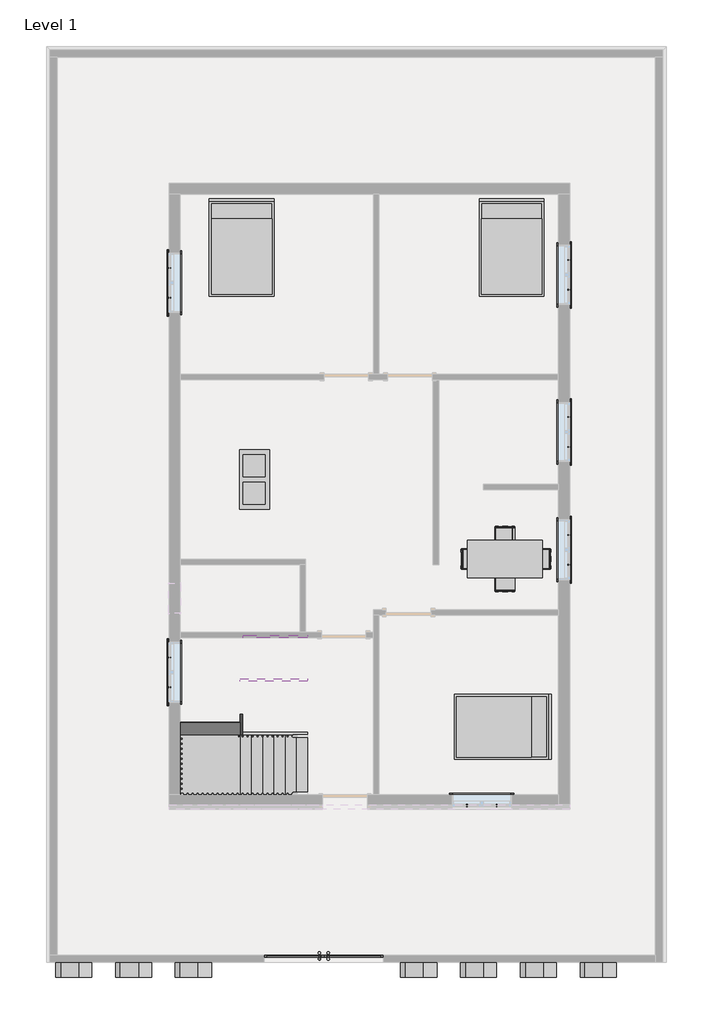
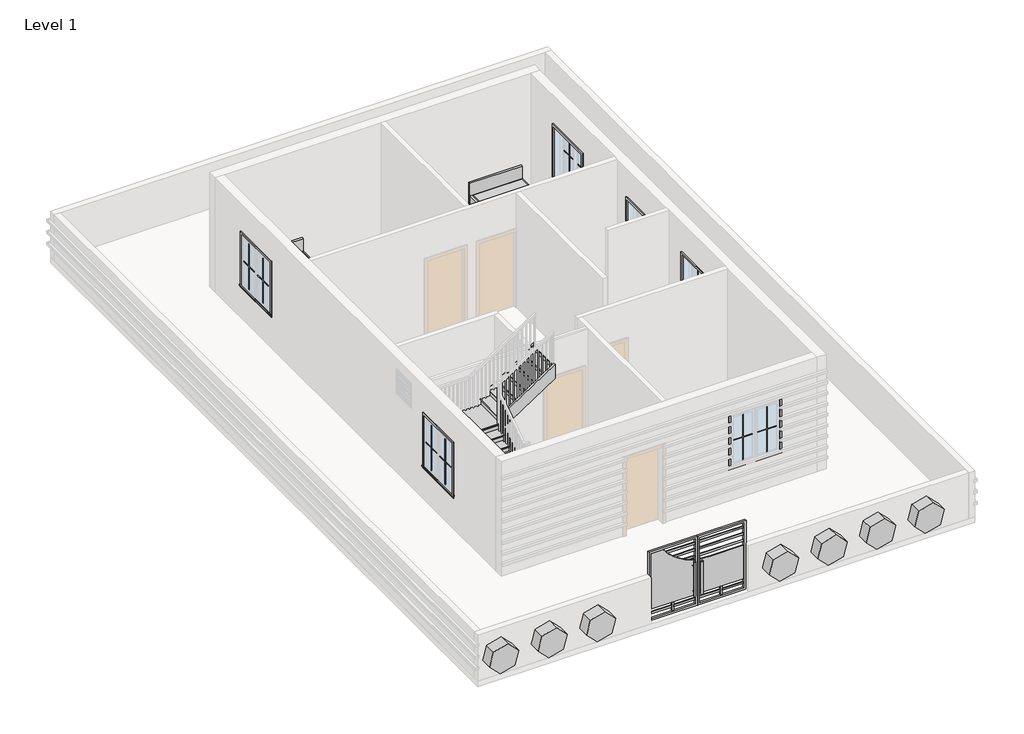
# One storey, part 4 of 4: 33 proxies, 5 members, 4 furniture elements, 1 stair flight.
"""IFC4 building model written with IfcOpenShell, lengths in millimetres."""

from ifc_helpers import new_model, si_unit, frame, origin, place, context, project, spatial, polyline, outline, extrude, transform, mapped, element, save
from components import generic_models_113f6068, generic_models_1_generic_models_1_b34c57ae, generic_models_2_generic_models_1_f357a12c, muntin_pattern_2x2_muntin_pattern_2x2_ba8901dc, muntin_pattern_2x2_muntin_pattern_2x2_877df4e9, trim_window_exterior_flat_with_sill_fda35bc9, trim_window_interior_flat_picture_frame_a80dbcd9, coffee_table_with_brass_mullions_11320_coffee_table_with_5962bef7, bed_17739_bed_17739_15c61121, dining_table_w_chairs_11374_0cdfc61b, stair_flight_6293cd8f

model = new_model("IFC4")

# Units and contexts
model_context = context("Model", 3, world=origin())
ifc_project = project(units=[si_unit("LENGTHUNIT", "METRE", prefix="MILLI")], contexts=[model_context])

# Site, building, storey
site = spatial("IfcSite", under=ifc_project)
building = spatial("IfcBuilding", under=site)
storey = spatial("IfcBuildingStorey", under=building, Name="Level 1", Elevation=0.0)

# Proxies
placement = place(None, origin())
generic_models_shape = generic_models_113f6068(model_context)
element("IfcBuildingElementProxy", 1, Name="Generic Models", at=placement, inside=storey, context=model_context, shape_type="MappedRepresentation", body=[
    mapped(generic_models_shape, transform((-2178.6617403, -9645.3989753, 0.0), x_axis=(1.0, 0.0, 0.0), y_axis=(0.0, 1.0, 0.0), z_axis=(0.0, 0.0, 1.0))),
])
generic_models_1_generic_models_1_shape = generic_models_1_generic_models_1_b34c57ae(model_context)
element("IfcBuildingElementProxy", 2, Name="Generic Models 1 : Generic Models 1", ObjectType="Generic Models 1 : Generic Models 1", at=placement, inside=storey, context=model_context, shape_type="MappedRepresentation", body=[
    mapped(generic_models_1_generic_models_1_shape, transform((0.0, 0.0, 0.0), x_axis=(1.0, 0.0, 0.0), y_axis=(0.0, 1.0, 0.0), z_axis=(0.0, 0.0, 1.0))),
])
generic_models_2_generic_models_1_shape = generic_models_2_generic_models_1_f357a12c(model_context)
element("IfcBuildingElementProxy", 3, Name="Generic Models 2 : Generic Models 1", ObjectType="Generic Models 2 : Generic Models 1", at=placement, inside=storey, context=model_context, shape_type="MappedRepresentation", body=[
    mapped(generic_models_2_generic_models_1_shape, transform((0.0, 0.0, 0.0), x_axis=(1.0, 0.0, 0.0), y_axis=(0.0, 1.0, 0.0), z_axis=(0.0, 0.0, 1.0))),
])
element("IfcBuildingElementProxy", 4, Name="Generic Models 3 : Generic Models 1", ObjectType="Generic Models 3 : Generic Models 1", at=placement, inside=storey, context=model_context, shape_type="MappedRepresentation", body=[
    mapped(generic_models_1_generic_models_1_shape, transform((2438.4, 0.0, 0.0), x_axis=(1.0, 0.0, 0.0), y_axis=(0.0, 1.0, 0.0), z_axis=(0.0, 0.0, 1.0))),
])
element("IfcBuildingElementProxy", 5, Name="Generic Models 4 : Generic Models 1", ObjectType="Generic Models 4 : Generic Models 1", at=placement, inside=storey, context=model_context, shape_type="MappedRepresentation", body=[
    mapped(generic_models_1_generic_models_1_shape, transform((7032.1849448, 0.0, 0.0), x_axis=(1.0, 0.0, 0.0), y_axis=(0.0, 1.0, 0.0), z_axis=(0.0, 0.0, 1.0))),
])
element("IfcBuildingElementProxy", 6, Name="Generic Models 5 : Generic Models 1", ObjectType="Generic Models 5 : Generic Models 1", at=placement, inside=storey, context=model_context, shape_type="MappedRepresentation", body=[
    mapped(generic_models_1_generic_models_1_shape, transform((8251.3849448, 0.0, 0.0), x_axis=(1.0, 0.0, 0.0), y_axis=(0.0, 1.0, 0.0), z_axis=(0.0, 0.0, 1.0))),
])
element("IfcBuildingElementProxy", 7, Name="Generic Models 6 : Generic Models 1", ObjectType="Generic Models 6 : Generic Models 1", at=placement, inside=storey, context=model_context, shape_type="MappedRepresentation", body=[
    mapped(generic_models_1_generic_models_1_shape, transform((9470.5849448, 0.0, 0.0), x_axis=(1.0, 0.0, 0.0), y_axis=(0.0, 1.0, 0.0), z_axis=(0.0, 0.0, 1.0))),
])
element("IfcBuildingElementProxy", 8, Name="Generic Models 7 : Generic Models 1", ObjectType="Generic Models 7 : Generic Models 1", at=placement, inside=storey, context=model_context, shape_type="MappedRepresentation", body=[
    mapped(generic_models_1_generic_models_1_shape, transform((10689.7849448, 0.0, 0.0), x_axis=(1.0, 0.0, 0.0), y_axis=(0.0, 1.0, 0.0), z_axis=(0.0, 0.0, 1.0))),
])
muntin_pattern_2x2_muntin_pattern_2x2_shape = muntin_pattern_2x2_muntin_pattern_2x2_ba8901dc(model_context)
element("IfcBuildingElementProxy", 9, Name="Muntin Pattern_2x2 : Muntin Pattern_2x2", ObjectType="Muntin Pattern_2x2 : Muntin Pattern_2x2", at=placement, inside=storey, context=model_context, shape_type="MappedRepresentation", body=[
    mapped(muntin_pattern_2x2_muntin_pattern_2x2_shape, transform((-5325.0867403, -4189.9051559, 984.25), x_axis=(0.0, 1.0, 0.0), y_axis=(-1.0, 0.0, 0.0), z_axis=(0.0, 0.0, 1.0))),
])
element("IfcBuildingElementProxy", 10, Name="Muntin Pattern_2x2 : Muntin Pattern_2x2", ObjectType="Muntin Pattern_2x2 : Muntin Pattern_2x2", at=placement, inside=storey, context=model_context, shape_type="MappedRepresentation", body=[
    mapped(muntin_pattern_2x2_muntin_pattern_2x2_shape, transform((-5325.0867403, 3744.4198441, 984.25), x_axis=(0.0, 1.0, 0.0), y_axis=(-1.0, 0.0, 0.0), z_axis=(0.0, 0.0, 1.0))),
])
element("IfcBuildingElementProxy", 11, Name="Muntin Pattern_2x2 : Muntin Pattern_2x2", ObjectType="Muntin Pattern_2x2 : Muntin Pattern_2x2", at=placement, inside=storey, context=model_context, shape_type="MappedRepresentation", body=[
    mapped(muntin_pattern_2x2_muntin_pattern_2x2_shape, transform((2821.9632597, 4512.7698441, 984.25), x_axis=(0.0, -1.0, 0.0), y_axis=(1.0, 0.0, 0.0), z_axis=(0.0, 0.0, 1.0))),
])
element("IfcBuildingElementProxy", 12, Name="Muntin Pattern_2x2 : Muntin Pattern_2x2", ObjectType="Muntin Pattern_2x2 : Muntin Pattern_2x2", at=placement, inside=storey, context=model_context, shape_type="MappedRepresentation", body=[
    mapped(muntin_pattern_2x2_muntin_pattern_2x2_shape, transform((2821.9632597, 1312.3698441, 984.25), x_axis=(0.0, -1.0, 0.0), y_axis=(1.0, 0.0, 0.0), z_axis=(0.0, 0.0, 1.0))),
])
element("IfcBuildingElementProxy", 13, Name="Muntin Pattern_2x2 : Muntin Pattern_2x2", ObjectType="Muntin Pattern_2x2 : Muntin Pattern_2x2", at=placement, inside=storey, context=model_context, shape_type="MappedRepresentation", body=[
    mapped(muntin_pattern_2x2_muntin_pattern_2x2_shape, transform((2821.9632597, -1087.9301559, 984.25), x_axis=(0.0, -1.0, 0.0), y_axis=(1.0, 0.0, 0.0), z_axis=(0.0, 0.0, 1.0))),
])
element("IfcBuildingElementProxy", 14, Name="Muntin Pattern_2x2 : Muntin Pattern_2x2", ObjectType="Muntin Pattern_2x2 : Muntin Pattern_2x2", at=placement, inside=storey, context=model_context, shape_type="MappedRepresentation", body=[
    mapped(muntin_pattern_2x2_muntin_pattern_2x2_shape, transform((1344.0007597, -6601.3176559, 984.25), x_axis=(-1.0, 0.0, 0.0), y_axis=(0.0, -1.0, 0.0), z_axis=(0.0, 0.0, 1.0))),
])
muntin_pattern_2x2_muntin_pattern_2x2_2_shape = muntin_pattern_2x2_muntin_pattern_2x2_877df4e9(model_context)
element("IfcBuildingElementProxy", 15, Name="Muntin Pattern_2x2 : Muntin Pattern_2x2", ObjectType="Muntin Pattern_2x2 : Muntin Pattern_2x2", at=placement, inside=storey, context=model_context, shape_type="MappedRepresentation", body=[
    mapped(muntin_pattern_2x2_muntin_pattern_2x2_2_shape, transform((-5325.0867403, -3583.4801559, 984.25), x_axis=(0.0, -1.0, 0.0), y_axis=(1.0, 0.0, 0.0), z_axis=(0.0, 0.0, 1.0))),
])
element("IfcBuildingElementProxy", 16, Name="Muntin Pattern_2x2 : Muntin Pattern_2x2", ObjectType="Muntin Pattern_2x2 : Muntin Pattern_2x2", at=placement, inside=storey, context=model_context, shape_type="MappedRepresentation", body=[
    mapped(muntin_pattern_2x2_muntin_pattern_2x2_2_shape, transform((-5325.0867403, 4350.8448441, 984.25), x_axis=(0.0, -1.0, 0.0), y_axis=(1.0, 0.0, 0.0), z_axis=(0.0, 0.0, 1.0))),
])
element("IfcBuildingElementProxy", 17, Name="Muntin Pattern_2x2 : Muntin Pattern_2x2", ObjectType="Muntin Pattern_2x2 : Muntin Pattern_2x2", at=placement, inside=storey, context=model_context, shape_type="MappedRepresentation", body=[
    mapped(muntin_pattern_2x2_muntin_pattern_2x2_2_shape, transform((2821.9632597, 3906.3448441, 984.25), x_axis=(0.0, 1.0, 0.0), y_axis=(-1.0, 0.0, 0.0), z_axis=(0.0, 0.0, 1.0))),
])
element("IfcBuildingElementProxy", 18, Name="Muntin Pattern_2x2 : Muntin Pattern_2x2", ObjectType="Muntin Pattern_2x2 : Muntin Pattern_2x2", at=placement, inside=storey, context=model_context, shape_type="MappedRepresentation", body=[
    mapped(muntin_pattern_2x2_muntin_pattern_2x2_2_shape, transform((2821.9632597, 705.9448441, 984.25), x_axis=(0.0, 1.0, 0.0), y_axis=(-1.0, 0.0, 0.0), z_axis=(0.0, 0.0, 1.0))),
])
element("IfcBuildingElementProxy", 19, Name="Muntin Pattern_2x2 : Muntin Pattern_2x2", ObjectType="Muntin Pattern_2x2 : Muntin Pattern_2x2", at=placement, inside=storey, context=model_context, shape_type="MappedRepresentation", body=[
    mapped(muntin_pattern_2x2_muntin_pattern_2x2_2_shape, transform((2821.9632597, -1694.3551559, 984.25), x_axis=(0.0, 1.0, 0.0), y_axis=(-1.0, 0.0, 0.0), z_axis=(0.0, 0.0, 1.0))),
])
element("IfcBuildingElementProxy", 20, Name="Muntin Pattern_2x2 : Muntin Pattern_2x2", ObjectType="Muntin Pattern_2x2 : Muntin Pattern_2x2", at=placement, inside=storey, context=model_context, shape_type="MappedRepresentation", body=[
    mapped(muntin_pattern_2x2_muntin_pattern_2x2_2_shape, transform((737.5757597, -6601.3176559, 984.25), x_axis=(1.0, 0.0, 0.0), y_axis=(0.0, 1.0, 0.0), z_axis=(0.0, 0.0, 1.0))),
])
trim_window_exterior_flat_with_sill_shape = trim_window_exterior_flat_with_sill_fda35bc9(model_context)
element("IfcBuildingElementProxy", 21, Name="Trim-Window-Exterior-Flat : with Sill", ObjectType="Trim-Window-Exterior-Flat : with Sill", at=placement, inside=storey, context=model_context, shape_type="MappedRepresentation", body=[
    mapped(trim_window_exterior_flat_with_sill_shape, transform((-5334.6117403, -3886.6926559, 2260.6), x_axis=(0.0, -1.0, 0.0), y_axis=(0.0, 0.0, 1.0), z_axis=(-1.0, 0.0, 0.0))),
])
element("IfcBuildingElementProxy", 22, Name="Trim-Window-Exterior-Flat : with Sill", ObjectType="Trim-Window-Exterior-Flat : with Sill", at=placement, inside=storey, context=model_context, shape_type="MappedRepresentation", body=[
    mapped(trim_window_exterior_flat_with_sill_shape, transform((-5334.6117403, 4047.6323441, 2260.6), x_axis=(0.0, -1.0, 0.0), y_axis=(0.0, 0.0, 1.0), z_axis=(-1.0, 0.0, 0.0))),
])
element("IfcBuildingElementProxy", 23, Name="Trim-Window-Exterior-Flat : with Sill", ObjectType="Trim-Window-Exterior-Flat : with Sill", at=placement, inside=storey, context=model_context, shape_type="MappedRepresentation", body=[
    mapped(trim_window_exterior_flat_with_sill_shape, transform((2831.4882597, 4209.5573441, 2260.6), x_axis=(0.0, 1.0, 0.0), y_axis=(0.0, 0.0, 1.0), z_axis=(1.0, 0.0, 0.0))),
])
element("IfcBuildingElementProxy", 24, Name="Trim-Window-Exterior-Flat : with Sill", ObjectType="Trim-Window-Exterior-Flat : with Sill", at=placement, inside=storey, context=model_context, shape_type="MappedRepresentation", body=[
    mapped(trim_window_exterior_flat_with_sill_shape, transform((2831.4882597, 1009.1573441, 2260.6), x_axis=(0.0, 1.0, 0.0), y_axis=(0.0, 0.0, 1.0), z_axis=(1.0, 0.0, 0.0))),
])
element("IfcBuildingElementProxy", 25, Name="Trim-Window-Exterior-Flat : with Sill", ObjectType="Trim-Window-Exterior-Flat : with Sill", at=placement, inside=storey, context=model_context, shape_type="MappedRepresentation", body=[
    mapped(trim_window_exterior_flat_with_sill_shape, transform((2831.4882597, -1391.1426559, 2260.6), x_axis=(0.0, 1.0, 0.0), y_axis=(0.0, 0.0, 1.0), z_axis=(1.0, 0.0, 0.0))),
])
element("IfcBuildingElementProxy", 26, Name="Trim-Window-Exterior-Flat : with Sill", ObjectType="Trim-Window-Exterior-Flat : with Sill", at=placement, inside=storey, context=model_context, shape_type="MappedRepresentation", body=[
    mapped(trim_window_exterior_flat_with_sill_shape, transform((1040.7882597, -6610.8426559, 2260.6), x_axis=(1.0, 0.0, 0.0), y_axis=(0.0, 0.0, 1.0), z_axis=(0.0, -1.0, 0.0))),
])
trim_window_interior_flat_picture_frame_shape = trim_window_interior_flat_picture_frame_a80dbcd9(model_context)
element("IfcBuildingElementProxy", 27, Name="Trim-Window-Interior-Flat : Picture Frame", ObjectType="Trim-Window-Interior-Flat : Picture Frame", at=placement, inside=storey, context=model_context, shape_type="MappedRepresentation", body=[
    mapped(trim_window_interior_flat_picture_frame_shape, transform((-5106.0117403, -3886.6926559, 2260.6), x_axis=(0.0, 1.0, 0.0), y_axis=(0.0, 0.0, 1.0), z_axis=(1.0, 0.0, 0.0))),
])
element("IfcBuildingElementProxy", 28, Name="Trim-Window-Interior-Flat : Picture Frame", ObjectType="Trim-Window-Interior-Flat : Picture Frame", at=placement, inside=storey, context=model_context, shape_type="MappedRepresentation", body=[
    mapped(trim_window_interior_flat_picture_frame_shape, transform((-5106.0117403, 4047.6323441, 2260.6), x_axis=(0.0, 1.0, 0.0), y_axis=(0.0, 0.0, 1.0), z_axis=(1.0, 0.0, 0.0))),
])
element("IfcBuildingElementProxy", 29, Name="Trim-Window-Interior-Flat : Picture Frame", ObjectType="Trim-Window-Interior-Flat : Picture Frame", at=placement, inside=storey, context=model_context, shape_type="MappedRepresentation", body=[
    mapped(trim_window_interior_flat_picture_frame_shape, transform((2602.8882597, 4209.5573441, 2260.6), x_axis=(0.0, -1.0, 0.0), y_axis=(0.0, 0.0, 1.0), z_axis=(-1.0, 0.0, 0.0))),
])
element("IfcBuildingElementProxy", 30, Name="Trim-Window-Interior-Flat : Picture Frame", ObjectType="Trim-Window-Interior-Flat : Picture Frame", at=placement, inside=storey, context=model_context, shape_type="MappedRepresentation", body=[
    mapped(trim_window_interior_flat_picture_frame_shape, transform((2602.8882597, 1009.1573441, 2260.6), x_axis=(0.0, -1.0, 0.0), y_axis=(0.0, 0.0, 1.0), z_axis=(-1.0, 0.0, 0.0))),
])
element("IfcBuildingElementProxy", 31, Name="Trim-Window-Interior-Flat : Picture Frame", ObjectType="Trim-Window-Interior-Flat : Picture Frame", at=placement, inside=storey, context=model_context, shape_type="MappedRepresentation", body=[
    mapped(trim_window_interior_flat_picture_frame_shape, transform((2602.8882597, -1391.1426559, 2260.6), x_axis=(0.0, -1.0, 0.0), y_axis=(0.0, 0.0, 1.0), z_axis=(-1.0, 0.0, 0.0))),
])
element("IfcBuildingElementProxy", 32, Name="Trim-Window-Interior-Flat : Picture Frame", ObjectType="Trim-Window-Interior-Flat : Picture Frame", at=placement, inside=storey, context=model_context, shape_type="MappedRepresentation", body=[
    mapped(trim_window_interior_flat_picture_frame_shape, transform((1040.7882597, -6382.2426559, 2260.6), x_axis=(-1.0, 0.0, 0.0), y_axis=(0.0, 0.0, 1.0), z_axis=(0.0, 1.0, 0.0))),
])
coffee_table_with_brass_mullions_11320_coffee_table_with_shape = coffee_table_with_brass_mullions_11320_coffee_table_with_5962bef7(model_context)
element("IfcBuildingElementProxy", 33, Name="coffee_table_with_brass_mullions_11320 : coffee_table_with_brass_mullions_11320", ObjectType="coffee_table_with_brass_mullions_11320 : coffee_table_with_brass_mullions_11320", at=placement, inside=storey, context=model_context, shape_type="MappedRepresentation", body=[
    mapped(coffee_table_with_brass_mullions_11320_coffee_table_with_shape, transform((-3162.9117403, 678.9573441, 0.0), x_axis=(0.0, 1.0, 0.0), y_axis=(-1.0, 0.0, 0.0), z_axis=(0.0, 0.0, 1.0))),
])

# Furniture
bed_17739_bed_17739_shape = bed_17739_bed_17739_15c61121(model_context)
element("IfcFurniture", 34, ObjectType="Bed_17739 : Bed_17739", at=placement, inside=storey, context=model_context, shape_type="MappedRepresentation", body=[
    mapped(bed_17739_bed_17739_shape, transform((-3855.0617403, 4742.9573441, 0.0), x_axis=(1.0, 0.0, 0.0), y_axis=(0.0, 1.0, 0.0), z_axis=(0.0, 0.0, 1.0))),
])
element("IfcFurniture", 35, ObjectType="Bed_17739 : Bed_17739", at=placement, inside=storey, context=model_context, shape_type="MappedRepresentation", body=[
    mapped(bed_17739_bed_17739_shape, transform((1650.3882597, 4742.9573441, 0.0), x_axis=(1.0, 0.0, 0.0), y_axis=(0.0, 1.0, 0.0), z_axis=(0.0, 0.0, 1.0))),
])
element("IfcFurniture", 36, ObjectType="Bed_17739 : Bed_17739", at=placement, inside=storey, context=model_context, shape_type="MappedRepresentation", body=[
    mapped(bed_17739_bed_17739_shape, transform((1447.1882597, -4997.9426559, 0.0), x_axis=(0.0, -1.0, 0.0), y_axis=(1.0, 0.0, 0.0), z_axis=(0.0, 0.0, 1.0))),
])
dining_table_w_chairs_11374_shape = dining_table_w_chairs_11374_0cdfc61b(model_context)
element("IfcFurniture", 37, ObjectType="Dining_Table_w_Chairs_11374", at=placement, inside=storey, context=model_context, shape_type="MappedRepresentation", body=[
    mapped(dining_table_w_chairs_11374_shape, transform((1497.0410232, -1671.6886654, 0.0), x_axis=(1.0, 0.0, 0.0), y_axis=(0.0, 1.0, 0.0), z_axis=(0.0, 0.0, 1.0))),
])

# Members
element("IfcMember", 38, ObjectType="Stringer - 2\" Width", at=placement, inside=storey, context=model_context, shape_type="SweptSolid", body=[
    extrude(outline(polyline([(0.0, -2515.2117403), (218.0398409, -2515.2117403), (472.0398409, -2896.2117403), (472.0398409, -3445.6977546), (0.0, -2737.6379933), (0.0, -2515.2117403)])), frame((0.0, -6433.0426559, 0.0), z_axis=(0.0, 1.0, 0.0), x_axis=(0.0, 0.0, 1.0)), (0.0, 0.0, 1.0), 50.8),
])
element("IfcMember", 39, ObjectType="Stringer - 2\" Width", at=placement, inside=storey, context=model_context, shape_type="SweptSolid", body=[
    extrude(outline(polyline([(2239.3158313, -3277.2117403), (2747.3158313, -2515.2117403), (3113.6398409, -2515.2117403), (2239.3158313, -3826.6977546), (2239.3158313, -3277.2117403)])), frame((0.0, -3181.8426559, 0.0), z_axis=(0.0, 1.0, 0.0), x_axis=(0.0, 0.0, 1.0)), (0.0, 0.0, 1.0), 50.8),
])
element("IfcMember", 40, ObjectType="Stringer - 2\" Width", at=placement, inside=storey, context=model_context, shape_type="SweptSolid", body=[
    extrude(outline(polyline([(0.0, -2515.2117403), (218.0398409, -2515.2117403), (1098.5731743, -3836.0117403), (732.2491647, -3836.0117403), (0.0, -2737.6379933), (0.0, -2515.2117403)])), frame((0.0, -5163.0426559, 0.0), z_axis=(0.0, 1.0, 0.0), x_axis=(0.0, 0.0, 1.0)), (0.0, 0.0, 1.0), 50.8),
])
element("IfcMember", 41, ObjectType="Stringer - 2\" Width", at=placement, inside=storey, context=model_context, shape_type="SweptSolid", body=[
    extrude(outline(polyline([(-5163.0426559, 918.5158313), (-5163.0426559, 1284.8398409), (-4070.8426559, 2012.9731743), (-4070.8426559, 1646.6491647), (-5163.0426559, 918.5158313)])), frame((-3886.8117403, 0.0, 0.0), z_axis=(1.0, 0.0, 0.0), x_axis=(0.0, 1.0, 0.0)), (0.0, 0.0, 1.0), 50.8),
])
element("IfcMember", 42, ObjectType="Stringer - 2\" Width", at=placement, inside=storey, context=model_context, shape_type="SweptSolid", body=[
    extrude(outline(polyline([(2199.2398409, -3886.8117403), (1832.9158313, -3886.8117403), (2747.3158313, -2515.2117403), (3113.6398409, -2515.2117403), (2199.2398409, -3886.8117403)])), frame((0.0, -4070.8426559, 0.0), z_axis=(0.0, 1.0, 0.0), x_axis=(0.0, 0.0, 1.0)), (0.0, 0.0, 1.0), 50.8),
])

# Stair flight
stair_flight_shape = stair_flight_6293cd8f(model_context)
element("IfcStairFlight", 43, ObjectType="2\" Tread 1\" Nosing 1/4\" Riser", at=placement, inside=storey, context=model_context, shape_type="MappedRepresentation", body=[
    mapped(stair_flight_shape, transform((0.0, 0.0, 0.0), x_axis=(1.0, 0.0, 0.0), y_axis=(0.0, 1.0, 0.0), z_axis=(0.0, 0.0, 1.0))),
])

save(model, "model.ifc")

# Revit data of these elements
# Type
#   sheet = none
#   pipe = none
#   handal = none
#   faram = none
#   Default Elevation = 0
# Type "Muntin Pattern_2x2 : Muntin Pattern_2x2"
#   Width [instance default] = 4' - 0"
#   Thickness = 0' - 0 1/2"
#   Height [instance default] = 4' - 0"
#   Distance = 0' - 0 3/4"
#   Interior Material [instance default] = none
#   Exterior Material [instance default] = none
#   Default Elevation = 0
# Type "Trim-Window-Exterior-Flat : with Sill"
#   Trim Width = 0' - 2 1/4"
#   Trim Thickness_Picture Frame = 0' - 1 1/4"
#   Trim Thickness_with Sill = 0' - 0 3/4"
#   Sill Thickness = 0' - 1 1/4"
#   Opening Width [instance default] = 2' - 0"
#   Opening Height [instance default] = 3' - 0"
#   Default Elevation = 4' - 0"
#   Sill = yes
#   Picture Frame = no
#   Trim Material [instance default] = none
# Type "Trim-Window-Interior-Flat : Picture Frame"
#   Trim Thickness_Picture Frame = 0' - 1 1/4"
#   Trim Width = 0' - 2 1/4"
#   Trim Thickness_with Sill = 0' - 0 3/4"
#   Sill Thickness = 0' - 1 1/4"
#   Opening Width [instance default] = 2' - 0"
#   Opening Height [instance default] = 3' - 0"
#   Default Elevation = 4' - 0"
#   Sill = no
#   Picture Frame = yes
#   Trim Material [instance default] = none
# Type "coffee_table_with_brass_mullions_11320 : coffee_table_with_brass_mullions_11320"
#   Default Elevation = 0
# Type "Bed_17739 : Bed_17739"
#   Default Elevation = 0
# Type "Dining_Table_w_Chairs_11374"
#   Default Elevation = 0
#   Assembly Code = ""
# Element 1 (IfcBuildingElementProxy)
#   Phase Created = New Construction
# Element 2 (IfcBuildingElementProxy, "Generic Models 1 : Generic Models 1")
#   Phase Created = New Construction
# Element 3 (IfcBuildingElementProxy, "Generic Models 2 : Generic Models 1")
#   Phase Created = New Construction
#   Materials on its faces: "Carpet (1)"
# Element 4 (IfcBuildingElementProxy, "Generic Models 3 : Generic Models 1")
#   Phase Created = New Construction
# Element 5 (IfcBuildingElementProxy, "Generic Models 4 : Generic Models 1")
#   Phase Created = New Construction
# Element 6 (IfcBuildingElementProxy, "Generic Models 5 : Generic Models 1")
#   Phase Created = New Construction
# Element 7 (IfcBuildingElementProxy, "Generic Models 6 : Generic Models 1")
#   Phase Created = New Construction
# Element 8 (IfcBuildingElementProxy, "Generic Models 7 : Generic Models 1")
#   Phase Created = New Construction
# Elements 9, 10, 11, 12, 13, 14, 15, 16, 17, 18, 19, 20 (IfcBuildingElementProxy, "Muntin Pattern_2x2 : Muntin Pattern_2x2")
#   Width = 1' - 6 5/8"
#   Height = 3' - 11 1/2"
#   Interior Material = Wood - Stained
#   Exterior Material = Clad - White
#   Phase Created = New Construction
#   Materials on its faces: "Clad - White", "Wood - Stained"
# Elements 21, 22, 23, 24, 25, 26 (IfcBuildingElementProxy, "Trim-Window-Exterior-Flat : with Sill")
#   Opening Width = 4' - 0"
#   Opening Height = 4' - 5"
#   Trim Material = Clad - White
#   Phase Created = New Construction
#   Materials on its faces: "Clad - White"
# Elements 27, 28, 29, 30, 31, 32 (IfcBuildingElementProxy, "Trim-Window-Interior-Flat : Picture Frame")
#   Opening Width = 4' - 0"
#   Opening Height = 4' - 5"
#   Trim Material = Wood - Stained
#   Phase Created = New Construction
#   Materials on its faces: "Wood - Stained"
# Element 33 (IfcBuildingElementProxy, "coffee_table_with_brass_mullions_11320 : coffee_table_with_brass_mullions_11320")
#   Phase Created = New Construction
#   Materials on its faces: "Default Wall", "TABLE", "Glass", "Default"
# Elements 34, 35, 36 (IfcFurniture, "Bed_17739 : Bed_17739")
#   Phase Created = New Construction
#   Materials on its faces: "legs", "sheets", "bed frame", "Blanket"
# Element 37 (IfcFurniture, "Dining_Table_w_Chairs_11374")
#   Phase Created = New Construction
# Elements 38, 39, 40, 41, 42 (IfcMember, "Stringer - 2\" Width")
#   Phase Created = New Construction
# Element 43 (IfcStairFlight, "2\" Tread 1\" Nosing 1/4\" Riser")
#   Phase Created = New Construction
#   Materials on its faces: "Wood Planks"
# Materials
#   "Carpet (1)": class "Carpet", colour RGB 124 80 67, transparency 0, Description = "Interior finish", Cost = 0
#   "Clad - White": class "Wood", colour RGB 242 242 238, transparency 0, Cost = 0
#   "Wood - Stained": class "Wood", colour RGB 224 178 126, transparency 0, Cost = 0
#   "Default Wall": colour RGB 128 128 128, transparency 0, Cost = 0
#   "TABLE": class "Generic", colour RGB 120 120 120, transparency 0, Cost = 0
#   "Glass": class "Glass", colour RGB 0 128 192, transparency 0.75, Description = "Soda Lime Glass", Cost = 0
#   "Default": colour RGB 127 127 127, transparency 0, Cost = 0
#   "legs": colour RGB 90 73 37, transparency 0, Cost = 0
#   "sheets": colour RGB 200 195 176, transparency 0, Cost = 0
#   "bed frame": colour RGB 90 73 37, transparency 0, Cost = 0
#   "Blanket": class "System", colour RGB 59 0 1, transparency 0, Cost = 0
#   "Wood Planks": class "Wood", colour RGB 193 160 115, transparency 0, Description = "Physical material.", Cost = 0
